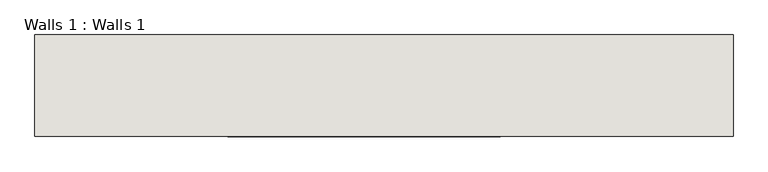
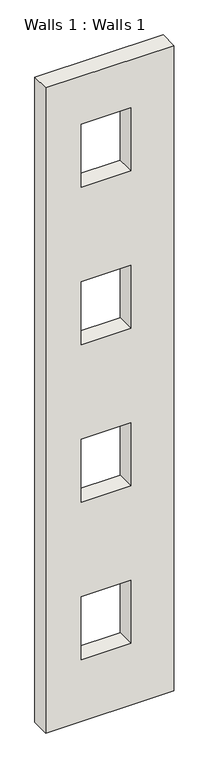
"""IFC4 building model written with IfcOpenShell, lengths in millimetres: wall geometry, Walls 1 : Walls 1."""

from ifc_helpers import new_model, si_unit, frame, origin, place, context, project, spatial, polyline, outline, extrude, source, transform, mapped, element, save


def walls_1_walls_1_8f4806b2(model_context):
    return source(origin(), model_context, "Body", "SweptSolid", [
        extrude(outline(polyline([(15233.65, 172.3175011), (2747.0724171, 172.3175011), (2747.0724171, 2517.5430349), (15233.65, 2517.5430349), (15233.65, 172.3175011)]), holes=[polyline([(3937.0, 820.7073388), (5156.2, 820.7073388), (5156.2, 1735.1073388), (3937.0, 1735.1073388), (3937.0, 820.7073388)]), polyline([(14300.2, 1735.1073388), (13081.0, 1735.1073388), (13081.0, 820.7073388), (14300.2, 820.7073388), (14300.2, 1735.1073388)]), polyline([(8204.2, 1735.1073388), (6985.0, 1735.1073388), (6985.0, 820.7073388), (8204.2, 820.7073388), (8204.2, 1735.1073388)]), polyline([(11252.2, 1735.1073388), (10033.0, 1735.1073388), (10033.0, 820.7073388), (11252.2, 820.7073388), (11252.2, 1735.1073388)])]), frame((0.0, 111.2788005, 0.0), z_axis=(0.0, 1.0, 0.0), x_axis=(0.0, 0.0, 1.0)), (0.0, 0.0, 1.0), 340.2267137),
    ])


if __name__ == "__main__":
    model = new_model("IFC4")
    model_context = context("Model", 3, world=origin())
    ifc_project = project(units=[si_unit("LENGTHUNIT", "METRE", prefix="MILLI")], contexts=[model_context])
    site = spatial("IfcSite", under=ifc_project)
    building = spatial("IfcBuilding", under=site)
    placement = place(None, origin())
    walls_1_walls_1_shape = walls_1_walls_1_8f4806b2(model_context)
    element("IfcWall", 1, ObjectType="Walls 1 : Walls 1", at=placement, inside=building, context=model_context, shape_type="MappedRepresentation", body=[
        mapped(walls_1_walls_1_shape, transform((0.0, 0.0, 0.0), x_axis=(1.0, 0.0, 0.0), y_axis=(0.0, 1.0, 0.0), z_axis=(0.0, 0.0, 1.0))),
    ])
    save(model, "model.ifc")

# Revit data of these elements
# Element 1 (IfcWall, "Walls 1 : Walls 1")
#   Materials on its faces: "1 wall brown", "Default Wall"
# Materials
#   "1 wall brown": class "Generic", colour RGB 61 46 37, transparency 0, Cost = 0
#   "Default Wall": colour RGB 128 128 128, transparency 0, Cost = 0
